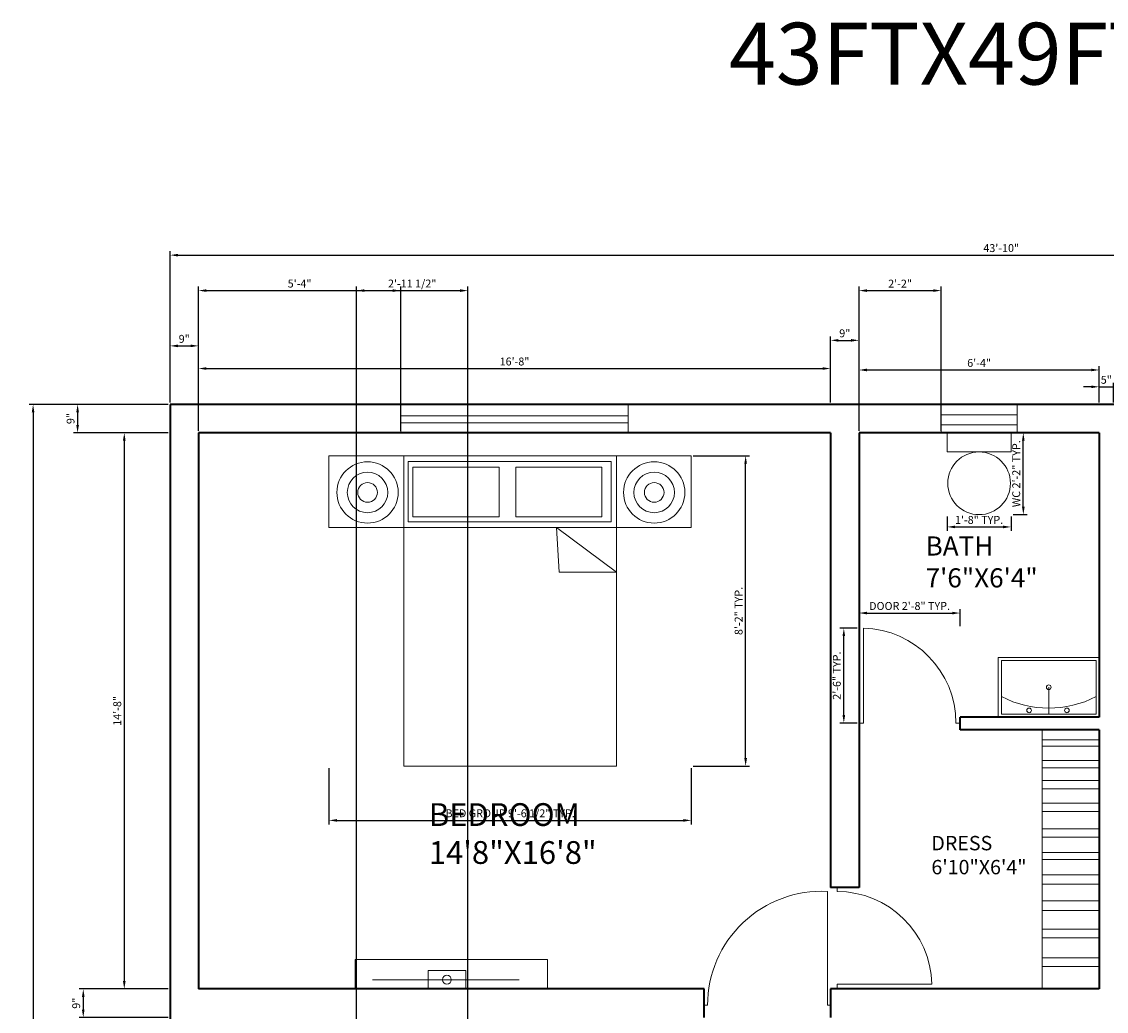
# Model space of a CAD drawing. Units: inches. Extents: x 808 to 1433, y 803 to 1556.
# Tile 3 of 4: x 808 to 1151, y 1243 to 1556. Entities that reach past the tile are written whole.
import ezdxf

# ---------------------------------------------------------------- set-up
doc = ezdxf.new("R2010")
doc.units = ezdxf.units.IN
for name, color, linetype, lineweight in [('A-ANNO-DIMS', 7, 'Continuous', 13), ('A-AREA-IDEN', 7, 'Continuous', 18), ('A-FLOR-CASE', 7, 'Continuous', 18), ('A-WALL', 7, 'Continuous', 35)]:
    doc.layers.add(name, color=color, linetype=linetype, lineweight=lineweight)
for name, color, linetype, lineweight, true_color in [('A-ANNO-TITL', 244, 'Continuous', 25, 0x991b1e), ('A-DOOR', 251, 'Continuous', 18, 0x636466), ('A-FLOR-FIXT', 251, 'Continuous', 18, 0x636466), ('A-FURN', 251, 'Continuous', 13, 0x636466), ('A-GLAZ', 251, 'Continuous', 18, 0x636466)]:
    doc.layers.add(name, color=color, linetype=linetype, lineweight=lineweight, true_color=true_color)
doc.styles.get("Standard").update_dxf_attribs({"font": 'arial.ttf'})
doc.dimstyles.new('ISO-25', dxfattribs={"dimtxt": 2.5, "dimasz": 2.5, "dimexe": 1.25, "dimexo": 0.625, "dimtad": 1, "dimdec": 0, "dimlunit": 3, "dimtxsty": 'Standard', "dimcen": 2.5, "dimadec": 0, "dimazin": 0, "dimtfac": 1, "dimtdec": 0, "dimtmove": 0, "dimatfit": 3, "dimfxl": 1, "dimarcsym": 0})

# ---------------------------------------------------------------- blocks, each defined once
blk = doc.blocks.new('*D1')
at = {"layer": 'A-ANNO-DIMS', "color": 0, "lineweight": -2, "transparency": 16777216}
for p, q in [((854.88, 1435.69), (854.88, 1483.54)), ((1380.88, 1435.69), (1380.88, 1483.54)), ((857.38, 1482.29), (1378.38, 1482.29))]:
    blk.add_line(p, q, dxfattribs=at)
at = {"layer": 'A-ANNO-DIMS', "color": 0, "transparency": 16777216}
for points in [[(857.38, 1482.7), (857.38, 1481.87), (854.88, 1482.29)], [(1378.38, 1482.7), (1378.38, 1481.87), (1380.88, 1482.29)]]:
    blk.add_solid(points, dxfattribs=at)
at = {"layer": 'Defpoints', "color": 0, "transparency": 16777216}
for p in [(1380.88, 1482.29), (854.88, 1435.07), (1380.88, 1435.07)]:
    blk.add_point(p, dxfattribs=at)
at = {"layer": 'A-ANNO-DIMS', "color": 0, "transparency": 16777216, "insert": (1117.88, 1484.19), "char_height": 2.5, "attachment_point": 5}
blk.add_mtext('43\'-10"', dxfattribs=at)
blk = doc.blocks.new('*D3')
at = {"layer": 'A-ANNO-DIMS', "color": 0, "lineweight": -2, "transparency": 16777216}
for p, q in [((854.88, 1435.69), (854.88, 1454.83)), ((857.38, 1453.58), (861.38, 1453.58)), ((863.88, 1435.69), (863.88, 1454.83))]:
    blk.add_line(p, q, dxfattribs=at)
at = {"layer": 'A-ANNO-DIMS', "color": 0, "transparency": 16777216}
for points in [[(857.38, 1453.99), (857.38, 1453.16), (854.88, 1453.58)], [(861.38, 1453.99), (861.38, 1453.16), (863.88, 1453.58)]]:
    blk.add_solid(points, dxfattribs=at)
at = {"layer": 'Defpoints', "color": 0, "transparency": 16777216}
for p in [(863.88, 1453.58), (854.88, 1435.07), (863.88, 1435.07)]:
    blk.add_point(p, dxfattribs=at)
at = {"layer": 'A-ANNO-DIMS', "color": 0, "transparency": 16777216, "insert": (859.38, 1455.48), "char_height": 2.5, "attachment_point": 5}
blk.add_mtext('9"', dxfattribs=at)
blk = doc.blocks.new('*D4')
at = {"layer": 'A-ANNO-DIMS', "color": 0, "lineweight": -2, "transparency": 16777216}
for p, q in [((863.88, 1435.69), (863.88, 1447.66)), ((866.38, 1446.41), (1061.38, 1446.41)), ((1063.88, 1435.69), (1063.88, 1447.66))]:
    blk.add_line(p, q, dxfattribs=at)
at = {"layer": 'A-ANNO-DIMS', "color": 0, "transparency": 16777216}
for points in [[(866.38, 1446.82), (866.38, 1445.99), (863.88, 1446.41)], [(1061.38, 1446.82), (1061.38, 1445.99), (1063.88, 1446.41)]]:
    blk.add_solid(points, dxfattribs=at)
at = {"layer": 'Defpoints', "color": 0, "transparency": 16777216}
for p in [(1063.88, 1446.41), (863.88, 1435.07), (1063.88, 1435.07)]:
    blk.add_point(p, dxfattribs=at)
at = {"layer": 'A-ANNO-DIMS', "color": 0, "transparency": 16777216, "insert": (963.88, 1448.31), "char_height": 2.5, "attachment_point": 5}
blk.add_mtext('16\'-8"', dxfattribs=at)
blk = doc.blocks.new('*D5')
at = {"layer": 'A-ANNO-DIMS', "color": 0, "lineweight": -2, "transparency": 16777216}
for p, q in [((1063.88, 1435.69), (1063.88, 1456.58)), ((1066.38, 1455.33), (1070.38, 1455.33)), ((1072.88, 1435.69), (1072.88, 1456.58))]:
    blk.add_line(p, q, dxfattribs=at)
at = {"layer": 'A-ANNO-DIMS', "color": 0, "transparency": 16777216}
for points in [[(1066.38, 1455.75), (1066.38, 1454.91), (1063.88, 1455.33)], [(1070.38, 1455.75), (1070.38, 1454.91), (1072.88, 1455.33)]]:
    blk.add_solid(points, dxfattribs=at)
at = {"layer": 'Defpoints', "color": 0, "transparency": 16777216}
for p in [(1072.88, 1455.33), (1063.88, 1435.07), (1072.88, 1435.07)]:
    blk.add_point(p, dxfattribs=at)
at = {"layer": 'A-ANNO-DIMS', "color": 0, "transparency": 16777216, "insert": (1068.38, 1457.23), "char_height": 2.5, "attachment_point": 5}
blk.add_mtext('9"', dxfattribs=at)
blk = doc.blocks.new('*D6')
at = {"layer": 'A-ANNO-DIMS', "color": 0, "lineweight": -2, "transparency": 16777216}
for p, q in [((1072.88, 1435.69), (1072.88, 1447.2)), ((1075.38, 1445.95), (1146.38, 1445.95)), ((1148.88, 1435.69), (1148.88, 1447.2))]:
    blk.add_line(p, q, dxfattribs=at)
at = {"layer": 'A-ANNO-DIMS', "color": 0, "transparency": 16777216}
for points in [[(1075.38, 1446.37), (1075.38, 1445.53), (1072.88, 1445.95)], [(1146.38, 1446.37), (1146.38, 1445.53), (1148.88, 1445.95)]]:
    blk.add_solid(points, dxfattribs=at)
at = {"layer": 'Defpoints', "color": 0, "transparency": 16777216}
for p in [(1148.88, 1445.95), (1072.88, 1435.07), (1148.88, 1435.07)]:
    blk.add_point(p, dxfattribs=at)
at = {"layer": 'A-ANNO-DIMS', "color": 0, "transparency": 16777216, "insert": (1110.88, 1447.85), "char_height": 2.5, "attachment_point": 5}
blk.add_mtext('6\'-4"', dxfattribs=at)
blk = doc.blocks.new('*D7')
at = {"layer": 'A-ANNO-DIMS', "color": 0, "lineweight": -2, "transparency": 16777216}
for p, q in [((1148.88, 1435.69), (1148.88, 1441.87)), ((1153.38, 1435.69), (1153.38, 1441.87)), ((1146.38, 1440.62), (1143.88, 1440.62)), ((1148.88, 1440.62), (1153.38, 1440.62)), ((1155.88, 1440.62), (1158.38, 1440.62))]:
    blk.add_line(p, q, dxfattribs=at)
at = {"layer": 'A-ANNO-DIMS', "color": 0, "transparency": 16777216}
for points in [[(1146.38, 1441.04), (1146.38, 1440.2), (1148.88, 1440.62)], [(1155.88, 1441.04), (1155.88, 1440.2), (1153.38, 1440.62)]]:
    blk.add_solid(points, dxfattribs=at)
at = {"layer": 'Defpoints', "color": 0, "transparency": 16777216}
for p in [(1153.38, 1440.62), (1148.88, 1435.07), (1153.38, 1435.07)]:
    blk.add_point(p, dxfattribs=at)
at = {"layer": 'A-ANNO-DIMS', "color": 0, "transparency": 16777216, "insert": (1151.13, 1442.52), "char_height": 2.5, "attachment_point": 5}
blk.add_mtext('5"', dxfattribs=at)
blk = doc.blocks.new('*D12')
at = {"layer": 'A-ANNO-DIMS', "color": 0, "lineweight": -2, "transparency": 16777216}
for p, q in [((854.25, 1435.07), (810.3, 1435.07)), ((811.55, 1432.57), (811.55, 843.57)), ((854.25, 841.07), (810.3, 841.07))]:
    blk.add_line(p, q, dxfattribs=at)
at = {"layer": 'A-ANNO-DIMS', "color": 0, "transparency": 16777216}
for points in [[(811.14, 1432.57), (811.97, 1432.57), (811.55, 1435.07)], [(811.14, 843.57), (811.97, 843.57), (811.55, 841.07)]]:
    blk.add_solid(points, dxfattribs=at)
at = {"layer": 'Defpoints', "color": 0, "transparency": 16777216}
for p in [(854.88, 1435.07), (811.55, 841.07), (854.88, 841.07)]:
    blk.add_point(p, dxfattribs=at)
at = {"layer": 'A-ANNO-DIMS', "color": 0, "transparency": 16777216, "insert": (809.65, 1138.07), "char_height": 2.5, "attachment_point": 5, "rotation": 90}
blk.add_mtext('49\'-6"', dxfattribs=at)
blk = doc.blocks.new('*D13')
at = {"layer": 'A-ANNO-DIMS', "color": 0, "lineweight": -2, "transparency": 16777216}
for p, q in [((854.25, 1435.07), (824.39, 1435.07)), ((825.64, 1432.57), (825.64, 1428.57)), ((854.25, 1426.07), (824.39, 1426.07))]:
    blk.add_line(p, q, dxfattribs=at)
at = {"layer": 'A-ANNO-DIMS', "color": 0, "transparency": 16777216}
for points in [[(825.22, 1432.57), (826.06, 1432.57), (825.64, 1435.07)], [(825.22, 1428.57), (826.06, 1428.57), (825.64, 1426.07)]]:
    blk.add_solid(points, dxfattribs=at)
at = {"layer": 'Defpoints', "color": 0, "transparency": 16777216}
for p in [(854.88, 1435.07), (825.64, 1426.07), (854.88, 1426.07)]:
    blk.add_point(p, dxfattribs=at)
at = {"layer": 'A-ANNO-DIMS', "color": 0, "transparency": 16777216, "insert": (823.74, 1430.57), "char_height": 2.5, "attachment_point": 5, "rotation": 90}
blk.add_mtext('9"', dxfattribs=at)
blk = doc.blocks.new('*D14')
at = {"layer": 'A-ANNO-DIMS', "color": 0, "lineweight": -2, "transparency": 16777216}
for p, q in [((854.25, 1426.07), (839.16, 1426.07)), ((840.41, 1423.57), (840.41, 1252.57)), ((854.25, 1250.07), (839.16, 1250.07))]:
    blk.add_line(p, q, dxfattribs=at)
at = {"layer": 'A-ANNO-DIMS', "color": 0, "transparency": 16777216}
for points in [[(839.99, 1423.57), (840.83, 1423.57), (840.41, 1426.07)], [(839.99, 1252.57), (840.83, 1252.57), (840.41, 1250.07)]]:
    blk.add_solid(points, dxfattribs=at)
at = {"layer": 'Defpoints', "color": 0, "transparency": 16777216}
for p in [(854.88, 1426.07), (840.41, 1250.07), (854.88, 1250.07)]:
    blk.add_point(p, dxfattribs=at)
at = {"layer": 'A-ANNO-DIMS', "color": 0, "transparency": 16777216, "insert": (838.51, 1338.07), "char_height": 2.5, "attachment_point": 5, "rotation": 90}
blk.add_mtext('14\'-8"', dxfattribs=at)
blk = doc.blocks.new('*D15')
at = {"layer": 'A-ANNO-DIMS', "color": 0, "lineweight": -2, "transparency": 16777216}
for p, q in [((854.25, 1250.07), (826.18, 1250.07)), ((827.43, 1247.57), (827.43, 1243.57)), ((854.25, 1241.07), (826.18, 1241.07))]:
    blk.add_line(p, q, dxfattribs=at)
at = {"layer": 'A-ANNO-DIMS', "color": 0, "transparency": 16777216}
for points in [[(827.01, 1247.57), (827.84, 1247.57), (827.43, 1250.07)], [(827.01, 1243.57), (827.84, 1243.57), (827.43, 1241.07)]]:
    blk.add_solid(points, dxfattribs=at)
at = {"layer": 'Defpoints', "color": 0, "transparency": 16777216}
for p in [(854.88, 1250.07), (827.43, 1241.07), (854.88, 1241.07)]:
    blk.add_point(p, dxfattribs=at)
at = {"layer": 'A-ANNO-DIMS', "color": 0, "transparency": 16777216, "insert": (825.52, 1245.57), "char_height": 2.5, "attachment_point": 5, "rotation": 90}
blk.add_mtext('9"', dxfattribs=at)
blk = doc.blocks.new('BED-DOUBLE-NIGHTSTANDS')
for p, q in [((23.66, 75.46), (90.98, 75.46)), ((72.01, 75.46), (90.98, 61.39)), ((72.82, 61.39), (72.01, 75.46)), ((90.98, 61.39), (72.82, 61.39))]:
    blk.add_line(p, q)
for points in [[(23.66, 98.16), (0, 98.16), (0, 75.46), (23.66, 75.46)], [(23.66, 0), (90.98, 0), (90.98, 98.16), (23.66, 98.16)], [(25.04, 77.24), (89.23, 77.24), (89.23, 96.41), (25.04, 96.41)], [(114.63, 98.16), (90.98, 98.16), (90.98, 75.46), (114.63, 75.46)], [(26.57, 78.89), (53.84, 78.89), (53.84, 94.57), (26.57, 94.57)], [(59.07, 78.89), (86.35, 78.89), (86.35, 94.57), (59.07, 94.57)]]:
    blk.add_lwpolyline(points, close=True)
for centre, radius in [((12.19, 86.58), 9.7), ((102.89, 86.58), 9.7), ((12.19, 86.58), 6.41), ((102.89, 86.58), 6.41), ((12.19, 86.58), 3.11), ((102.89, 86.58), 3.11)]:
    blk.add_circle(centre, radius)
blk = doc.blocks.new('MEDIA-CONSOLE')
for q in [(6.39, 51.9), (6.39, 5.5)]:
    blk.add_line((6.39, 23.14), q)
for points in [[(9.33, 60.92), (0, 60.92), (0, 0), (9.33, 0)], [(9.33, 35.01), (3.45, 35.01), (3.45, 23.14), (9.33, 23.14)]]:
    blk.add_lwpolyline(points, close=True)
blk.add_circle((6.39, 29.07), 1.39)
blk = doc.blocks.new('WC')
blk.add_lwpolyline([(0, 19.84), (20.21, 19.84), (20.21, 25.9), (0, 25.9)], close=True)
for start, end in [(90, 270), (270, 90)]:
    blk.add_arc((10.11, 9.92), 9.92, start, end)
blk = doc.blocks.new('WIN-72')
for points in [[(0, 0), (72, 0), (72, 9), (0, 9)], [(0, 5.39), (72, 5.39), (72, 3.12), (0, 3.12)]]:
    blk.add_lwpolyline(points, close=True)
blk = doc.blocks.new('WIN-24')
for p, q in [((0, 5.64), (24, 5.64)), ((0, 2.5), (24, 2.5))]:
    blk.add_line(p, q)
blk.add_lwpolyline([(0, 0), (24, 0), (24, 9), (0, 9)], close=True)
blk = doc.blocks.new('DOOR-32')
for p, q in [((1.38, 0), (1.38, 30)), ((1.38, 0), (0, 0)), ((32, 0), (30.69, 0))]:
    blk.add_line(p, q)
blk.add_arc((0.68, 0), 30.01, 0, 88.664)
blk = doc.blocks.new('DOOR-40')
for p, q in [((0, 40), (0, 38.9)), ((0, 1), (36, 1)), ((0, 1), (0, 0))]:
    blk.add_line(p, q)
blk.add_arc((0, 2.85), 36.05, 357.0527, 90)
blk = doc.blocks.new('*D45')
at = {"layer": 'A-ANNO-DIMS', "color": 0, "lineweight": -2, "transparency": 16777216}
for p, q in [((1072.88, 1364.85), (1072.88, 1370.28)), ((1104.88, 1364.85), (1104.88, 1370.28)), ((1075.38, 1369.03), (1102.38, 1369.03))]:
    blk.add_line(p, q, dxfattribs=at)
at = {"layer": 'A-ANNO-DIMS', "color": 0, "transparency": 16777216}
for points in [[(1075.38, 1369.44), (1075.38, 1368.61), (1072.88, 1369.03)], [(1102.38, 1369.44), (1102.38, 1368.61), (1104.88, 1369.03)]]:
    blk.add_solid(points, dxfattribs=at)
at = {"layer": 'Defpoints', "color": 0, "transparency": 16777216}
for p in [(1104.88, 1369.03), (1072.88, 1364.23), (1104.88, 1364.23)]:
    blk.add_point(p, dxfattribs=at)
at = {"layer": 'A-ANNO-DIMS', "color": 0, "transparency": 16777216, "insert": (1088.88, 1370.95), "char_height": 2.5, "attachment_point": 5}
blk.add_mtext('DOOR 2\'-8" TYP.', dxfattribs=at)
blk = doc.blocks.new('*D46')
at = {"layer": 'A-ANNO-DIMS', "color": 0, "lineweight": -2, "transparency": 16777216}
for p, q in [((1072.25, 1364.23), (1066.83, 1364.23)), ((1068.08, 1336.73), (1068.08, 1361.73)), ((1072.25, 1334.23), (1066.83, 1334.23))]:
    blk.add_line(p, q, dxfattribs=at)
at = {"layer": 'A-ANNO-DIMS', "color": 0, "transparency": 16777216}
for points in [[(1067.66, 1361.73), (1068.5, 1361.73), (1068.08, 1364.23)], [(1067.66, 1336.73), (1068.5, 1336.73), (1068.08, 1334.23)]]:
    blk.add_solid(points, dxfattribs=at)
at = {"layer": 'Defpoints', "color": 0, "transparency": 16777216}
for p in [(1068.08, 1364.23), (1072.88, 1364.23), (1072.88, 1334.23)]:
    blk.add_point(p, dxfattribs=at)
at = {"layer": 'A-ANNO-DIMS', "color": 0, "transparency": 16777216, "insert": (1066.18, 1349.23), "char_height": 2.5, "attachment_point": 5, "rotation": 90}
blk.add_mtext('2\'-6" TYP.', dxfattribs=at)
blk = doc.blocks.new('*D49')
at = {"layer": 'A-ANNO-DIMS', "color": 0, "lineweight": -2, "transparency": 16777216}
for p, q in [((905.18, 1319.99), (905.18, 1302.17)), ((1019.82, 1319.99), (1019.82, 1302.17)), ((907.68, 1303.42), (1017.32, 1303.42))]:
    blk.add_line(p, q, dxfattribs=at)
at = {"layer": 'A-ANNO-DIMS', "color": 0, "transparency": 16777216}
for points in [[(907.68, 1303.84), (907.68, 1303.01), (905.18, 1303.42)], [(1017.32, 1303.84), (1017.32, 1303.01), (1019.82, 1303.42)]]:
    blk.add_solid(points, dxfattribs=at)
at = {"layer": 'Defpoints', "color": 0, "transparency": 16777216}
for p in [(905.18, 1320.62), (1019.82, 1320.62), (1019.82, 1303.42)]:
    blk.add_point(p, dxfattribs=at)
at = {"layer": 'A-ANNO-DIMS', "color": 0, "transparency": 16777216, "insert": (962.5, 1305.34), "char_height": 2.5, "attachment_point": 5}
blk.add_mtext('BED GROUP 9\'-6 1/2" TYP.', dxfattribs=at)
blk = doc.blocks.new('*D50')
at = {"layer": 'A-ANNO-DIMS', "color": 0, "lineweight": -2, "transparency": 16777216}
for p, q in [((1020.44, 1418.78), (1038.26, 1418.78)), ((1037.01, 1323.12), (1037.01, 1416.28)), ((1020.44, 1320.62), (1038.26, 1320.62))]:
    blk.add_line(p, q, dxfattribs=at)
at = {"layer": 'A-ANNO-DIMS', "color": 0, "transparency": 16777216}
for points in [[(1036.59, 1416.28), (1037.43, 1416.28), (1037.01, 1418.78)], [(1036.59, 1323.12), (1037.43, 1323.12), (1037.01, 1320.62)]]:
    blk.add_solid(points, dxfattribs=at)
at = {"layer": 'Defpoints', "color": 0, "transparency": 16777216}
for p in [(1019.82, 1418.78), (1037.01, 1418.78), (1019.82, 1320.62)]:
    blk.add_point(p, dxfattribs=at)
at = {"layer": 'A-ANNO-DIMS', "color": 0, "transparency": 16777216, "insert": (1035.11, 1369.7), "char_height": 2.5, "attachment_point": 5, "rotation": 90}
blk.add_mtext('8\'-2" TYP.', dxfattribs=at)
blk = doc.blocks.new('*D51')
at = {"layer": 'A-ANNO-DIMS', "color": 0, "lineweight": -2, "transparency": 16777216}
for p, q in [((1121.61, 1426.07), (1126.12, 1426.07)), ((1124.87, 1402.67), (1124.87, 1423.57)), ((1121.61, 1400.17), (1126.12, 1400.17))]:
    blk.add_line(p, q, dxfattribs=at)
at = {"layer": 'A-ANNO-DIMS', "color": 0, "transparency": 16777216}
for points in [[(1124.45, 1423.57), (1125.29, 1423.57), (1124.87, 1426.07)], [(1124.45, 1402.67), (1125.29, 1402.67), (1124.87, 1400.17)]]:
    blk.add_solid(points, dxfattribs=at)
at = {"layer": 'Defpoints', "color": 0, "transparency": 16777216}
for p in [(1120.99, 1426.07), (1124.87, 1426.07), (1120.99, 1400.17)]:
    blk.add_point(p, dxfattribs=at)
at = {"layer": 'A-ANNO-DIMS', "color": 0, "transparency": 16777216, "insert": (1122.95, 1413.12), "char_height": 2.5, "attachment_point": 5, "rotation": 90}
blk.add_mtext('WC 2\'-2" TYP.', dxfattribs=at)
blk = doc.blocks.new('*D52')
at = {"layer": 'A-ANNO-DIMS', "color": 0, "lineweight": -2, "transparency": 16777216}
for p, q in [((1100.77, 1399.54), (1100.77, 1395.03)), ((1120.99, 1399.54), (1120.99, 1395.03)), ((1103.27, 1396.28), (1118.49, 1396.28))]:
    blk.add_line(p, q, dxfattribs=at)
at = {"layer": 'A-ANNO-DIMS', "color": 0, "transparency": 16777216}
for points in [[(1103.27, 1396.7), (1103.27, 1395.87), (1100.77, 1396.28)], [(1118.49, 1396.7), (1118.49, 1395.87), (1120.99, 1396.28)]]:
    blk.add_solid(points, dxfattribs=at)
at = {"layer": 'Defpoints', "color": 0, "transparency": 16777216}
for p in [(1100.77, 1400.17), (1120.99, 1400.17), (1120.99, 1396.28)]:
    blk.add_point(p, dxfattribs=at)
at = {"layer": 'A-ANNO-DIMS', "color": 0, "transparency": 16777216, "insert": (1110.88, 1398.18), "char_height": 2.5, "attachment_point": 5}
blk.add_mtext('1\'-8" TYP.', dxfattribs=at)
blk = doc.blocks.new('*D68')
at = {"layer": 'A-ANNO-DIMS', "color": 0, "lineweight": -2, "transparency": 16777216}
for p, q in [((863.88, 1426.69), (863.88, 1472.32)), ((927.88, 1426.69), (927.88, 1472.32)), ((866.38, 1471.07), (925.38, 1471.07))]:
    blk.add_line(p, q, dxfattribs=at)
at = {"layer": 'A-ANNO-DIMS', "color": 0, "transparency": 16777216}
for points in [[(866.38, 1471.48), (866.38, 1470.65), (863.88, 1471.07)], [(925.38, 1471.48), (925.38, 1470.65), (927.88, 1471.07)]]:
    blk.add_solid(points, dxfattribs=at)
at = {"layer": 'Defpoints', "color": 0, "transparency": 16777216}
for p in [(927.88, 1471.07), (863.88, 1426.07), (927.88, 1426.07)]:
    blk.add_point(p, dxfattribs=at)
at = {"layer": 'A-ANNO-DIMS', "color": 0, "transparency": 16777216, "insert": (895.88, 1472.96), "char_height": 2.5, "attachment_point": 5}
blk.add_mtext('5\'-4"', dxfattribs=at)
blk = doc.blocks.new('*D72')
at = {"layer": 'A-ANNO-DIMS', "color": 0, "lineweight": -2, "transparency": 16777216}
for p, q in [((1072.88, 1426.69), (1072.88, 1472.32)), ((1098.88, 1426.69), (1098.88, 1472.32)), ((1075.38, 1471.07), (1096.38, 1471.07))]:
    blk.add_line(p, q, dxfattribs=at)
at = {"layer": 'A-ANNO-DIMS', "color": 0, "transparency": 16777216}
for points in [[(1075.38, 1471.48), (1075.38, 1470.65), (1072.88, 1471.07)], [(1096.38, 1471.48), (1096.38, 1470.65), (1098.88, 1471.07)]]:
    blk.add_solid(points, dxfattribs=at)
at = {"layer": 'Defpoints', "color": 0, "transparency": 16777216}
for p in [(1098.88, 1471.07), (1072.88, 1426.07), (1098.88, 1426.07)]:
    blk.add_point(p, dxfattribs=at)
at = {"layer": 'A-ANNO-DIMS', "color": 0, "transparency": 16777216, "insert": (1085.88, 1472.95), "char_height": 2.5, "attachment_point": 5}
blk.add_mtext('2\'-2"', dxfattribs=at)
blk = doc.blocks.new('*D78')
at = {"layer": 'A-ANNO-DIMS', "color": 0, "lineweight": -2, "transparency": 16777216}
for p, q in [((913.88, 1102), (913.88, 1472.32)), ((949.15, 1102), (949.15, 1472.32)), ((916.38, 1471.07), (946.65, 1471.07))]:
    blk.add_line(p, q, dxfattribs=at)
at = {"layer": 'A-ANNO-DIMS', "color": 0, "transparency": 16777216}
for points in [[(916.38, 1471.48), (916.38, 1470.65), (913.88, 1471.07)], [(946.65, 1471.48), (946.65, 1470.65), (949.15, 1471.07)]]:
    blk.add_solid(points, dxfattribs=at)
at = {"layer": 'Defpoints', "color": 0, "transparency": 16777216}
for p in [(949.15, 1471.07), (913.88, 1101.37), (949.15, 1101.37)]:
    blk.add_point(p, dxfattribs=at)
at = {"layer": 'A-ANNO-DIMS', "color": 0, "transparency": 16777216, "insert": (931.51, 1472.98), "char_height": 2.5, "attachment_point": 5}
blk.add_mtext('2\'-11 1/2"', dxfattribs=at)

msp = doc.modelspace()

# ---------------------------------------------------------------- linework, layer by layer
at = {"layer": 'A-FLOR-CASE'}
for p, q in [((1130.88, 1332.07), (1130.88, 1250.07)), ((1130.88, 1328.86), (1148.88, 1328.86)), ((1130.88, 1326.91), (1148.88, 1326.91)), ((1130.88, 1322.38), (1148.88, 1322.38)), ((1130.88, 1320), (1148.88, 1320)), ((1130.88, 1316), (1148.88, 1316)), ((1130.88, 1313.38), (1148.88, 1313.38)), ((1130.88, 1308.82), (1148.88, 1308.82)), ((1130.88, 1306.19), (1148.88, 1306.19)), ((1130.88, 1300.74), (1148.88, 1300.74)), ((1130.88, 1298.12), (1148.88, 1298.12)), ((1130.88, 1293.29), (1148.88, 1293.29)), ((1130.88, 1291.07), (1148.88, 1291.07)), ((1130.88, 1286.19), (1148.88, 1286.19)), ((1130.88, 1283.24), (1148.88, 1283.24)), ((1130.88, 1277.96), (1148.88, 1277.96)), ((1130.88, 1274.88), (1148.88, 1274.88)), ((1130.88, 1268.97), (1148.88, 1268.97)), ((1130.88, 1266.27), (1148.88, 1266.27)), ((1130.88, 1259.91), (1148.88, 1259.91)), ((1130.88, 1257.2), (1148.88, 1257.2))]:
    msp.add_line(p, q, dxfattribs=at)
at = {"layer": 'A-FLOR-FIXT'}
msp.add_line((1132.91, 1337.07), (1132.91, 1345.54), dxfattribs=at)
for points in [[(1148.88, 1336.07), (1116.93, 1336.07), (1116.93, 1355.01), (1148.88, 1355.01)], [(1147.88, 1337.07), (1117.93, 1337.07), (1117.93, 1354.01), (1147.88, 1354.01)]]:
    msp.add_lwpolyline(points, close=True, dxfattribs=at)
for centre in [(1132.91, 1345.54), (1126.71, 1338.24), (1138.67, 1338.24)]:
    msp.add_circle(centre, 0.737, dxfattribs=at)
msp.add_arc((1132.91, 1371.41), 32.48, 242.5485, 297.4515, dxfattribs=at)
at = {"layer": 'A-WALL'}
for p, q in [((1380.88, 1435.07), (854.88, 1435.07)), ((854.88, 1435.07), (854.88, 841.07)), ((863.88, 1426.07), (863.88, 1250.07)), ((1063.88, 1426.07), (863.88, 1426.07)), ((1063.88, 1426.07), (1063.88, 1282.23)), ((1072.88, 1426.07), (1072.88, 1332.07)), ((1148.88, 1426.07), (1072.88, 1426.07)), ((1148.88, 1426.07), (1148.88, 1336.07)), ((1148.88, 1336.07), (1104.88, 1336.07)), ((1104.88, 1332.07), (1104.88, 1336.07)), ((1072.88, 1332.07), (1072.88, 1282.23)), ((1148.88, 1332.07), (1104.88, 1332.07)), ((1148.88, 1332.07), (1148.88, 1250.07)), ((1072.88, 1282.23), (1063.88, 1282.23)), ((1023.88, 1250.07), (863.88, 1250.07)), ((1023.88, 1241.07), (1023.88, 1250.07)), ((1148.88, 1250.07), (1063.88, 1250.07)), ((1063.88, 1250.07), (1063.88, 1241.07))]:
    msp.add_line(p, q, dxfattribs=at)

# ---------------------------------------------------------------- block references
at = {"layer": 'A-DOOR'}
msp.add_blockref('DOOR-32', (1072.88, 1334.23), dxfattribs=at)
at = {"layer": 'A-DOOR', "rotation": 90.00000000000234}
msp.add_blockref('DOOR-40', (1063.88, 1244.94), dxfattribs=at)
at = {"layer": 'A-DOOR', "extrusion": (0, 0, -1), "zscale": -1, "rotation": 89.99999999998948}
msp.add_blockref('DOOR-32', (-1065.93, 1250.23), dxfattribs=at)
at = {"layer": 'A-FLOR-FIXT'}
msp.add_blockref('WC', (1100.77, 1400.17), dxfattribs=at)
at = {"layer": 'A-FURN'}
msp.add_blockref('BED-DOUBLE-NIGHTSTANDS', (905.18, 1320.62), dxfattribs=at)
at = {"layer": 'A-FURN', "rotation": 270.0000000000009}
msp.add_blockref('MEDIA-CONSOLE', (913.42, 1259.4), dxfattribs=at)
at = {"layer": 'A-GLAZ'}
for name, p in [('WIN-72', (927.88, 1426.07)), ('WIN-24', (1098.88, 1426.07))]:
    msp.add_blockref(name, p, dxfattribs=at)

# ---------------------------------------------------------------- texts
at = {"layer": 'A-ANNO-TITL', "insert": (1031.76, 1555.82), "char_height": 19.557, "attachment_point": 1}
msp.add_mtext_dynamic_manual_height_columns('43FTX49FT', width=1471.4106, gutter_width=97.78, heights=[0], dxfattribs=at)
at = {"layer": 'A-AREA-IDEN', "attachment_point": 1}
for s, width, gutter_width, insert, char_height in [('BATH\\P7\'6"X6\'4"', 64.9083, 30.26, (1093.95, 1393.28), 6.051), ('BEDROOM\\P14\'8"X16\'8"', 312.5212, 36.01, (936.76, 1308.86), 7.2014), ('DRESS\\P6\'10"X6\'4"', 37.3514, 22.75, (1095.78, 1298.5), 4.55)]:
    msp.add_mtext_dynamic_manual_height_columns(s, width=width, gutter_width=gutter_width, heights=[0], dxfattribs=dict(at, insert=insert, char_height=char_height))

# ---------------------------------------------------------------- dimensions: what is measured, and where the dimension line sits
at = {"layer": 'A-ANNO-DIMS'}
for base, p1, p2, override, picture, middle in [((1380.88, 1482.29), (854.88, 1435.07), (1380.88, 1435.07), {"dimclrd": 0, "dimclre": 0, "dimclrt": 0}, '*D1', (1117.88, 1484.19)), ((949.15, 1471.07), (913.88, 1101.37), (949.15, 1101.37), {"dimdec": 1, "dimlfac": 1, "dimrnd": 0, "dimzin": 1, "dimdsep": 46, "dimlunit": 4, "dimfrac": 2}, '*D78', (931.51, 1472.98)), ((927.88, 1471.07), (863.88, 1426.07), (927.88, 1426.07), {"dimdec": 1, "dimlfac": 1, "dimrnd": 0, "dimzin": 1, "dimdsep": 46, "dimlunit": 4, "dimfrac": 2}, '*D68', (895.88, 1472.96)), ((1098.88, 1471.07), (1072.88, 1426.07), (1098.88, 1426.07), {"dimdec": 1, "dimlfac": 1, "dimrnd": 0, "dimzin": 1, "dimdsep": 46, "dimlunit": 4, "dimfrac": 2}, '*D72', (1085.88, 1472.95)), ((1072.88, 1455.33), (1063.88, 1435.07), (1072.88, 1435.07), {"dimclrd": 0, "dimclre": 0, "dimclrt": 0}, '*D5', (1068.38, 1457.23)), ((863.88, 1453.58), (854.88, 1435.07), (863.88, 1435.07), {"dimclrd": 0, "dimclre": 0, "dimclrt": 0}, '*D3', (859.38, 1455.48)), ((1063.88, 1446.41), (863.88, 1435.07), (1063.88, 1435.07), {"dimclrd": 0, "dimclre": 0, "dimclrt": 0}, '*D4', (963.88, 1448.31)), ((1148.88, 1445.95), (1072.88, 1435.07), (1148.88, 1435.07), {"dimclrd": 0, "dimclre": 0, "dimclrt": 0}, '*D6', (1110.88, 1447.85)), ((1153.37953788, 1440.61951025), (1148.87953788, 1435.06624021), (1153.37953788, 1435.06624021), {"dimclrd": 0, "dimclre": 0, "dimclrt": 0}, '*D7', (1151.12953788, 1442.51582676))]:
    dim = msp.add_linear_dim(base=base, p1=p1, p2=p2, dimstyle='ISO-25', override=override, dxfattribs=at)
    dim.commit()
    dim.dimension.update_dxf_attribs({"geometry": picture, "text_midpoint": middle})
for base, p1, p2, picture, middle in [((811.55, 841.07), (854.88, 1435.07), (854.88, 841.07), '*D12', (809.65, 1138.07)), ((825.64, 1426.07), (854.88, 1435.07), (854.88, 1426.07), '*D13', (823.74, 1430.57)), ((840.41, 1250.07), (854.88, 1426.07), (854.88, 1250.07), '*D14', (838.51, 1338.07)), ((827.43, 1241.07), (854.88, 1250.07), (854.88, 1241.07), '*D15', (825.52, 1245.57))]:
    dim = msp.add_linear_dim(base=base, p1=p1, p2=p2, angle=90, dimstyle='ISO-25', override={"dimclrd": 0, "dimclre": 0, "dimclrt": 0}, dxfattribs=at)
    dim.commit()
    dim.dimension.update_dxf_attribs({"geometry": picture, "text_midpoint": middle})
for base, p1, p2, text, picture, middle in [((1124.87, 1426.07), (1120.99, 1400.17), (1120.99, 1426.07), 'WC <> TYP.', '*D51', (1122.95, 1413.12)), ((1037.01, 1418.78), (1019.82, 1320.62), (1019.82, 1418.78), '<> TYP.', '*D50', (1035.11, 1369.7)), ((1068.08, 1364.23), (1072.88, 1334.23), (1072.88, 1364.23), '<> TYP.', '*D46', (1066.18, 1349.23))]:
    dim = msp.add_linear_dim(base=base, p1=p1, p2=p2, angle=90, text=text, dimstyle='ISO-25', override={"dimdec": 1, "dimlfac": 1, "dimrnd": 0, "dimzin": 1, "dimdsep": 46, "dimlunit": 4, "dimfrac": 2}, dxfattribs=at)
    dim.commit()
    dim.dimension.update_dxf_attribs({"geometry": picture, "text_midpoint": middle})
for base, p1, p2, text, picture, middle in [((1120.99, 1396.28), (1100.77, 1400.17), (1120.99, 1400.17), '<> TYP.', '*D52', (1110.88, 1398.18)), ((1104.88, 1369.03), (1072.88, 1364.23), (1104.88, 1364.23), 'DOOR <> TYP.', '*D45', (1088.88, 1370.95)), ((1019.82, 1303.42), (905.18, 1320.62), (1019.82, 1320.62), 'BED GROUP <> TYP.', '*D49', (962.5, 1305.34))]:
    dim = msp.add_linear_dim(base=base, p1=p1, p2=p2, text=text, dimstyle='ISO-25', override={"dimdec": 1, "dimlfac": 1, "dimrnd": 0, "dimzin": 1, "dimdsep": 46, "dimlunit": 4, "dimfrac": 2}, dxfattribs=at)
    dim.commit()
    dim.dimension.update_dxf_attribs({"geometry": picture, "text_midpoint": middle})

doc.saveas('drawing.dxf')
